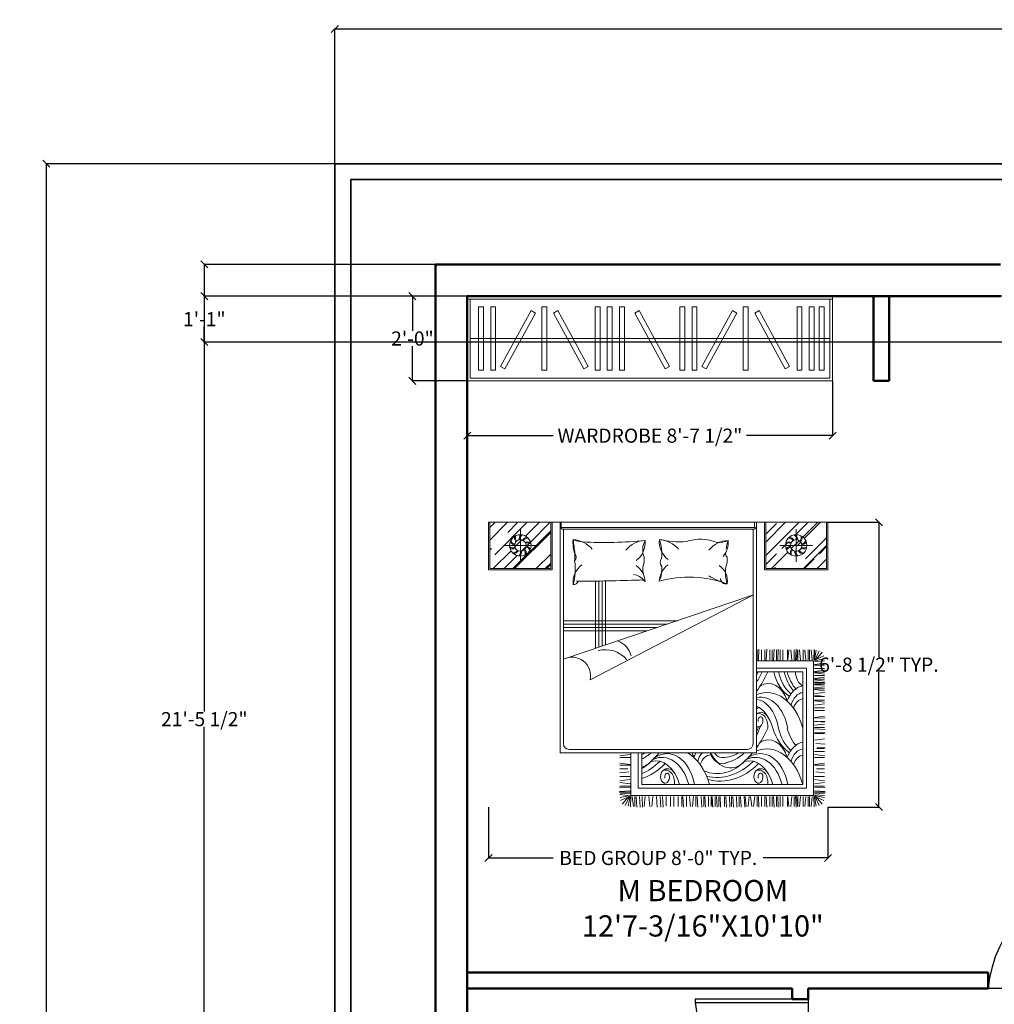
# Model space of a CAD drawing. Units: inches. Extents: x -317284 to 524, y -2236 to 1075.
# Tile 5 of 6: x -24 to 252, y 796 to 1075. Entities that reach past the tile are written whole.
import ezdxf

# ---------------------------------------------------------------- set-up
doc = ezdxf.new("R2010")
doc.units = ezdxf.units.IN
doc.header["$MEASUREMENT"] = 0
for name, color, linetype, lineweight in [('A-ANNO-DIMS', 2, 'Continuous', 18), ('A-AREA-IDEN', 7, 'Continuous', 18), ('A-DOOR', 4, 'Continuous', 25), ('A-FLOR-CASE', 8, 'Continuous', 20), ('A-FURN', 8, 'Continuous', 18), ('A-WALL', 7, 'Continuous', 50), ('C-PROP', 3, 'Continuous', 35)]:
    doc.layers.add(name, color=color, linetype=linetype, lineweight=lineweight)
doc.styles.get("Standard").update_dxf_attribs({"font": 'arial.ttf'})
doc.dimstyles.get("Standard").update_dxf_attribs({"dimtxt": 4, "dimasz": 2, "dimexe": 0.18, "dimexo": 0.0625, "dimgap": 0.09, "dimtad": 0, "dimtih": 1, "dimtoh": 1, "dimdec": 0, "dimzin": 0, "dimdsep": 46, "dimlunit": 4, "dimtxsty": 'Standard', "dimblk": 'OBLIQUE', "dimcen": 0.09, "dimadec": 0, "dimazin": 0, "dimtfac": 1, "dimtdec": 0, "dimtofl": 0, "dimtmove": 0, "dimatfit": 3, "dimldrblk": 'OBLIQUE', "dimfxl": 1, "dimtolj": 1, "dimtzin": 0, "dimarcsym": 0})

# ---------------------------------------------------------------- blocks, each defined once
blk = doc.blocks.new('SDFGHJK')
for p, q in [((282.73, 832.88), (281.73, 832.88)), ((281.73, 832.88), (281.73, 800.88)), ((282.73, 800.88), (282.73, 832.88)), ((282.73, 800.88), (250.73, 800.88))]:
    blk.add_line(p, q)
blk.add_arc((286.22, 797.51), 35.65, 97.2399, 174.5788)
blk = doc.blocks.new('A$C141F3920')
for p, q in [((600, 2590), (0, 2590)), ((0, 2590), (0, 0)), ((20, 0), (20, 2590)), ((600, 0), (600, 2590)), ((580, 2570), (20, 2570)), ((75, 2530.3), (75, 2495.3)), ((525, 2530.3), (75, 2530.3)), ((300, 20), (300, 2570)), ((525, 2495.3), (525, 2530.3)), ((580, 20), (580, 2570)), ((75, 2495.3), (525, 2495.3)), ((75, 2458.1), (75, 2423.1)), ((525, 2458.1), (75, 2458.1)), ((525, 2423.1), (525, 2458.1)), ((75, 2423.1), (525, 2423.1)), ((75, 2372.7), (75, 2337.7)), ((525, 2372.7), (75, 2372.7)), ((75, 2337.7), (525, 2337.7)), ((525, 2337.7), (525, 2372.7)), ((102.6, 2069.2), (497.4, 2285.1)), ((514.2, 2254.4), (119.4, 2038.5)), ((497.4, 2285.1), (514.2, 2254.4)), ((119.4, 2038.5), (102.6, 2069.2)), ((75, 1992), (75, 1957)), ((525, 1992), (75, 1992)), ((75, 1957), (525, 1957)), ((525, 1957), (525, 1992)), ((119.4, 1910.5), (102.6, 1879.8)), ((514.2, 1694.6), (119.4, 1910.5)), ((102.6, 1879.8), (497.4, 1663.9)), ((497.4, 1663.9), (514.2, 1694.6)), ((75, 1628.5), (75, 1593.5)), ((525, 1628.5), (75, 1628.5)), ((525, 1593.5), (525, 1628.5)), ((75, 1593.5), (525, 1593.5)), ((75, 1543.1), (75, 1508.1)), ((525, 1543.1), (75, 1543.1)), ((525, 1508.1), (525, 1543.1)), ((75, 1508.1), (525, 1508.1)), ((102.6, 1218.8), (497.4, 1434.8)), ((514.2, 1404), (119.4, 1188.1)), ((497.4, 1434.8), (514.2, 1404)), ((119.4, 1188.1), (102.6, 1218.8)), ((75, 1113.6), (75, 1078.6)), ((525, 1113.6), (75, 1113.6)), ((75, 1078.6), (525, 1078.6)), ((525, 1078.6), (525, 1113.6)), ((75, 1027.8), (75, 992.8)), ((525, 1027.8), (75, 1027.8)), ((75, 992.8), (525, 992.8)), ((525, 992.8), (525, 1027.8)), ((75, 942.3), (75, 907.3)), ((525, 942.3), (75, 942.3)), ((75, 907.3), (525, 907.3)), ((525, 907.3), (525, 942.3)), ((102.6, 641.9), (497.4, 857.9)), ((497.4, 857.9), (514.2, 827.2)), ((514.2, 827.2), (119.4, 611.2)), ((119.4, 611.2), (102.6, 641.9)), ((75, 564.8), (75, 529.8)), ((525, 564.8), (75, 564.8)), ((525, 529.8), (525, 564.8)), ((75, 529.8), (525, 529.8)), ((119.4, 483.3), (102.6, 452.6)), ((102.6, 452.6), (497.4, 236.7)), ((514.2, 267.4), (119.4, 483.3)), ((497.4, 236.7), (514.2, 267.4)), ((75, 201.3), (75, 166.3)), ((525, 201.3), (75, 201.3)), ((75, 166.3), (525, 166.3)), ((525, 166.3), (525, 201.3)), ((75, 115.8), (75, 80.8)), ((525, 115.8), (75, 115.8)), ((75, 80.8), (525, 80.8)), ((525, 80.8), (525, 115.8)), ((20, 20), (580, 20)), ((0, 0), (600, 0))]:
    blk.add_line(p, q)
blk = doc.blocks.new('A$C64B41DC1')
for p, q in [((0, 2.5079), (2.9903, 2.5079)), ((0, 2.0879), (0, 2.5079)), ((0.012, 2.4618), (0.0581, 2.5079)), ((0.012, 2.3515), (0.1684, 2.5079)), ((0.012, 2.0999), (0.012, 2.5079)), ((0.0543, 2.2213), (0.3409, 2.5079)), ((0.1689, 2.4179), (0.2589, 2.5079)), ((0.2157, 2.0999), (0.548, 2.4322)), ((0.2804, 2.1597), (0.2804, 2.4481)), ((0.3265, 2.386), (0.4484, 2.5079)), ((0.3699, 2.3332), (0.5445, 2.5079)), ((0.548, 2.5079), (0.548, 2.0999)), ((0.56, 2.5079), (0.56, 2.0879)), ((0.6301, 2.5079), (0.6301, 0.4779)), ((0.6401, 2.461), (0.6401, 2.5079)), ((0.6401, 2.5079), (2.344, 2.5079)), ((2.344, 2.461), (0.6401, 2.461)), ((0.6601, 2.4461), (1.4951, 2.4461)), ((0.6601, 2.4461), (0.6601, 0.5579)), ((1.4951, 2.4461), (0.6697, 2.4461)), ((2.3301, 2.4461), (1.4951, 2.4461)), ((2.3301, 0.5579), (2.3301, 2.4461)), ((2.344, 2.5079), (2.3601, 2.5079)), ((2.344, 2.5079), (2.344, 2.461)), ((2.3601, 2.5079), (2.3601, 2.4761)), ((2.3601, 0.4779), (2.3601, 2.5079)), ((2.4303, 2.5079), (2.4303, 2.0879)), ((2.4423, 2.5079), (2.4423, 2.0999)), ((2.4423, 2.3333), (2.6169, 2.5079)), ((2.4423, 2.2145), (2.7357, 2.5079)), ((2.4423, 2.404), (2.5354, 2.4971)), ((2.705, 2.398), (2.8149, 2.5079)), ((2.7099, 2.1597), (2.7099, 2.4481)), ((2.7691, 2.3772), (2.8998, 2.5079)), ((2.7819, 2.3646), (2.9252, 2.5079)), ((2.9783, 2.0999), (2.9783, 2.5079)), ((2.9903, 2.0879), (2.9903, 2.5079)), ((0.2299, 2.0999), (0.548, 2.418)), ((0.2311, 2.2906), (0.2937, 2.3532)), ((2.6674, 2.2756), (2.7382, 2.3464)), ((2.7914, 2.1846), (2.9783, 2.3715)), ((0.012, 2.261), (0.0275, 2.2765)), ((0.0404, 2.0999), (0.1982, 2.2578)), ((0.1362, 2.3039), (0.4246, 2.3039)), ((0.2905, 2.2539), (0.3304, 2.2938)), ((0.3405, 2.3039), (0.3605, 2.3238)), ((2.8541, 2.3039), (2.5657, 2.3039)), ((2.5849, 2.2779), (2.6158, 2.3088)), ((2.6158, 2.3088), (2.6313, 2.3243)), ((2.7249, 2.3076), (2.7512, 2.3339)), ((2.7746, 2.0999), (2.9783, 2.3036)), ((2.9144, 2.2312), (2.9783, 2.2951)), ((0.1365, 2.0999), (0.251, 2.2144)), ((0.4194, 2.0999), (0.548, 2.2285)), ((2.4423, 2.1353), (2.5382, 2.2312)), ((2.4918, 2.0999), (2.6366, 2.2447)), ((2.7831, 2.0999), (2.8678, 2.1846)), ((2.8962, 2.0999), (2.9783, 2.182)), ((0.56, 2.0879), (0, 2.0879)), ((0.548, 2.0999), (0.012, 2.0999)), ((0.4986, 2.0999), (0.548, 2.1493)), ((0.5127, 2.0999), (0.548, 2.1352)), ((2.4303, 2.0879), (2.9903, 2.0879)), ((2.4423, 2.0999), (2.9783, 2.0999)), ((2.5172, 2.0999), (2.5269, 2.1096)), ((0.9415, 1.9902), (0.9415, 1.3975)), ((0.9715, 1.9906), (0.9715, 1.4076)), ((1.0015, 1.991), (1.0015, 1.4177)), ((1.0315, 1.9916), (1.0315, 1.4279)), ((2.3349, 1.8678), (0.6613, 1.3029)), ((0.8956, 1.1191), (2.3349, 1.8678)), ((1.6636, 1.6412), (0.6601, 1.6412)), ((1.5748, 1.6112), (0.6601, 1.6112)), ((2.377, 1.295), (2.3822, 1.3891)), ((2.4451, 1.295), (2.4503, 1.3891)), ((2.5105, 1.295), (2.5157, 1.3891)), ((2.5471, 1.295), (2.5524, 1.3891)), ((2.7043, 1.295), (2.7095, 1.3891)), ((2.3665, 1.295), (2.3665, 1.3839)), ((2.4032, 1.295), (2.4032, 1.3839)), ((2.4346, 1.295), (2.4346, 1.3839)), ((2.4774, 1.2957), (2.4774, 1.3837)), ((2.5, 1.295), (2.5, 1.3839)), ((2.5367, 1.295), (2.5367, 1.3839)), ((2.5681, 1.295), (2.5681, 1.3839)), ((2.5918, 1.295), (2.5918, 1.3839)), ((2.6346, 1.2957), (2.6346, 1.3837)), ((2.6362, 1.2957), (2.6467, 1.3839)), ((2.6729, 1.295), (2.6624, 1.3839)), ((2.6938, 1.295), (2.6938, 1.3839)), ((2.7127, 1.2957), (2.7232, 1.3839)), ((2.7253, 1.295), (2.7253, 1.3839)), ((2.7494, 1.295), (2.7389, 1.3839)), ((2.7718, 1.295), (2.7718, 1.3839)), ((2.7959, 1.295), (2.7854, 1.3839)), ((2.8146, 1.2957), (2.8146, 1.3837)), ((2.8146, 1.2957), (2.8146, 1.3837)), ((2.8282, 1.295), (2.8282, 1.3839)), ((2.8282, 1.295), (2.8282, 1.3839)), ((2.8523, 1.295), (2.8418, 1.3839)), ((2.8523, 1.295), (2.8418, 1.3839)), ((2.8653, 1.2966), (2.8688, 1.3861)), ((2.8711, 1.2957), (2.8711, 1.3837)), ((2.8711, 1.2957), (2.8875, 1.3822)), ((2.8713, 1.2927), (2.954, 1.3315)), ((2.8717, 1.2884), (2.9588, 1.3058)), ((2.8765, 1.2958), (2.9132, 1.3758)), ((2.8893, 1.3011), (2.9394, 1.3636)), ((2.3601, 1.2873), (2.8639, 1.2873)), ((2.3601, 1.2233), (2.7999, 1.2233)), ((2.7999, 1.2233), (2.7999, 0.1658)), ((2.8639, 1.2873), (2.8639, 0.1018)), ((2.8716, 1.2565), (2.9605, 1.2669)), ((2.8716, 1.2212), (2.9605, 1.2212)), ((2.8723, 1.2489), (2.9603, 1.2489)), ((2.8744, 1.2817), (2.9603, 1.2869)), ((2.3601, 1.1913), (2.7679, 1.1912)), ((2.7679, 1.1912), (2.7679, 0.1978)), ((2.8716, 1.1947), (2.9605, 1.2052)), ((2.8716, 1.181), (2.9605, 1.1705)), ((2.8716, 1.1595), (2.9605, 1.1595)), ((2.8716, 1.133), (2.9605, 1.1435)), ((2.8723, 1.1872), (2.9603, 1.1872)), ((2.8716, 1.1193), (2.9605, 1.1088)), ((2.8716, 1.1035), (2.9605, 1.093)), ((2.8716, 1.0965), (2.9605, 1.0965)), ((2.8716, 1.086), (2.9657, 1.0913)), ((2.8716, 1.0756), (2.9605, 1.0756)), ((2.8716, 1.0491), (2.9605, 1.0596)), ((2.8723, 1.1255), (2.9603, 1.1255)), ((2.8723, 1.0858), (2.9605, 1.0753)), ((2.8723, 1.0416), (2.9603, 1.0416)), ((2.8716, 1.0354), (2.9605, 1.0249)), ((2.8723, 0.9987), (2.9605, 1.0092)), ((2.8723, 0.985), (2.9605, 0.9745)), ((2.8723, 0.9735), (2.9603, 0.9735)), ((2.8716, 0.9346), (2.9605, 0.9241)), ((2.8723, 0.9408), (2.9603, 0.9408)), ((2.8723, 0.8979), (2.9605, 0.9084)), ((2.8723, 0.8726), (2.9603, 0.8726)), ((2.8716, 0.7885), (2.9605, 0.799)), ((2.8716, 0.7818), (2.9657, 0.787)), ((2.8723, 0.8505), (2.9603, 0.8505)), ((2.8716, 0.7503), (2.9657, 0.7556)), ((2.8716, 0.7204), (2.9605, 0.7309)), ((2.8716, 0.6995), (2.9605, 0.6995)), ((2.8723, 0.7571), (2.9605, 0.7466)), ((2.8716, 0.689), (2.9657, 0.6838)), ((2.8716, 0.6576), (2.9657, 0.6523)), ((2.8716, 0.6471), (2.9605, 0.6471)), ((2.8716, 0.5903), (2.9605, 0.6007)), ((2.882, 0.5582), (2.9657, 0.5536)), ((2.8909, 0.5263), (2.9657, 0.5222)), ((0.6301, 0.4779), (2.3601, 0.4779)), ((0.7101, 0.5079), (2.2801, 0.5079)), ((1.2465, 0.4625), (1.1576, 0.452)), ((1.2465, 0.4365), (1.1577, 0.4365)), ((1.2542, 0.1018), (1.2542, 0.4779)), ((1.3182, 0.1658), (1.3182, 0.4779)), ((1.3502, 0.1978), (1.3502, 0.4779)), ((2.8716, 0.4877), (2.9603, 0.4877)), ((2.8716, 0.4625), (2.9605, 0.452)), ((2.8716, 0.4365), (2.9603, 0.4365)), ((2.8928, 0.5169), (2.9605, 0.5169)), ((1.2465, 0.3746), (1.1576, 0.3851)), ((1.2465, 0.3684), (1.1577, 0.3684)), ((2.8716, 0.3746), (2.9605, 0.3851)), ((2.8716, 0.3684), (2.9603, 0.3684)), ((1.2355, 0.3092), (1.1576, 0.3)), ((1.2285, 0.3357), (1.1577, 0.3357)), ((1.2457, 0.2676), (1.1577, 0.2676)), ((2.8723, 0.2676), (2.9603, 0.2676)), ((2.8826, 0.3092), (2.9605, 0.3)), ((2.8896, 0.3357), (2.9603, 0.3357)), ((1.2465, 0.1742), (1.1524, 0.169)), ((1.2457, 0.2423), (1.1576, 0.2319)), ((1.2465, 0.2057), (1.1576, 0.2161)), ((1.2465, 0.1847), (1.1576, 0.1847)), ((2.7679, 0.1978), (1.3502, 0.1978)), ((2.8716, 0.2057), (2.9605, 0.2161)), ((2.8716, 0.1847), (2.9605, 0.1847)), ((2.8716, 0.1742), (2.9657, 0.169)), ((2.8723, 0.2423), (2.9605, 0.2319)), ((1.2465, 0.1428), (1.1524, 0.1376)), ((1.2465, 0.1334), (1.1524, 0.1281)), ((1.2465, 0.1323), (1.1576, 0.1323)), ((1.2465, 0.1323), (1.1576, 0.1323)), ((1.2465, 0.1), (1.1576, 0.1105)), ((1.2465, 0.1229), (1.1588, 0.1168)), ((1.2464, 0.1007), (1.1592, 0.0833)), ((1.2468, 0.0964), (1.1641, 0.0576)), ((1.2288, 0.088), (1.1787, 0.0255)), ((1.2415, 0.0933), (1.2049, 0.0133)), ((1.247, 0.0934), (1.2306, 0.0069)), ((1.2527, 0.0925), (1.2493, 0.003)), ((2.8639, 0.1018), (1.2542, 0.1018)), ((1.2658, 0.0941), (1.2762, 0.0052)), ((1.2899, 0.0941), (1.2899, 0.0052)), ((1.2999, 0.0941), (1.3051, 0)), ((2.7999, 0.1658), (1.3182, 0.1658)), ((1.3313, 0.0941), (1.3365, 0)), ((1.3523, 0.0941), (1.3575, 0)), ((1.3804, 0.0941), (1.3699, 0.0052)), ((1.4119, 0.0934), (1.4223, 0.0052)), ((1.4485, 0.0941), (1.438, 0.0052)), ((1.48, 0.0941), (1.4852, 0)), ((1.5114, 0.0941), (1.5166, 0)), ((1.5323, 0.0941), (1.5376, 0)), ((1.5638, 0.0941), (1.5638, 0.0105)), ((1.6021, 0.0941), (1.6021, 0.0052)), ((1.6336, 0.0941), (1.6336, 0.0052)), ((1.6702, 0.0941), (1.6702, 0.0052)), ((1.7017, 0.0941), (1.7017, 0.0052)), ((1.7122, 0.0941), (1.7174, 0)), ((1.7445, 0.0934), (1.7445, 0.0054)), ((1.7698, 0.0934), (1.7803, 0.0052)), ((1.8065, 0.0941), (1.796, 0.0052)), ((1.8274, 0.0941), (1.8274, 0.0052)), ((1.8379, 0.0941), (1.8431, 0)), ((1.8746, 0.0941), (1.8798, 0)), ((1.8955, 0.0941), (1.8955, 0.0052)), ((1.906, 0.0941), (1.9113, 0)), ((1.9384, 0.0934), (1.9384, 0.0054)), ((1.9609, 0.0941), (1.9609, 0.0052)), ((1.9636, 0.0934), (1.9741, 0.0052)), ((1.9714, 0.0941), (1.9766, 0)), ((1.9976, 0.0941), (1.9976, 0.0052)), ((2.0081, 0.0941), (2.0133, 0)), ((2.029, 0.0941), (2.029, 0.0052)), ((2.0395, 0.0941), (2.0447, 0)), ((2.0797, 0.0941), (2.0797, 0.0052)), ((2.0902, 0.0941), (2.0954, 0)), ((2.1216, 0.0941), (2.1269, 0)), ((2.1412, 0.0941), (2.1412, 0.0052)), ((2.1517, 0.0941), (2.1569, 0)), ((2.1831, 0.0941), (2.1884, 0)), ((2.2093, 0.0941), (2.2093, 0.0052)), ((2.2198, 0.0941), (2.225, 0)), ((2.2512, 0.0941), (2.2565, 0)), ((2.2603, 0.0934), (2.2707, 0.0052)), ((2.2969, 0.0941), (2.2864, 0.0052)), ((2.3089, 0.0934), (2.3193, 0.0052)), ((2.3455, 0.0941), (2.3351, 0.0052)), ((2.3665, 0.0941), (2.3665, 0.0052)), ((2.377, 0.0941), (2.3822, 0)), ((2.4032, 0.0941), (2.4032, 0.0052)), ((2.4346, 0.0941), (2.4346, 0.0052)), ((2.4451, 0.0941), (2.4503, 0)), ((2.4774, 0.0934), (2.4774, 0.0054)), ((2.5, 0.0941), (2.5, 0.0052)), ((2.5105, 0.0941), (2.5157, 0)), ((2.5367, 0.0941), (2.5367, 0.0052)), ((2.5471, 0.0941), (2.5524, 0)), ((2.5681, 0.0941), (2.5681, 0.0052)), ((2.5918, 0.0941), (2.5918, 0.0052)), ((2.6346, 0.0934), (2.6346, 0.0054)), ((2.6362, 0.0934), (2.6467, 0.0052)), ((2.6729, 0.0941), (2.6624, 0.0052)), ((2.6938, 0.0941), (2.6938, 0.0052)), ((2.7043, 0.0941), (2.7095, 0)), ((2.7127, 0.0934), (2.7232, 0.0052)), ((2.7253, 0.0941), (2.7253, 0.0052)), ((2.7494, 0.0941), (2.7389, 0.0052)), ((2.7718, 0.0941), (2.7718, 0.0052)), ((2.7959, 0.0941), (2.7854, 0.0052)), ((2.8146, 0.0934), (2.8146, 0.0054)), ((2.8282, 0.0941), (2.8282, 0.0052)), ((2.8523, 0.0941), (2.8418, 0.0052)), ((2.8653, 0.0925), (2.8688, 0.003)), ((2.8711, 0.0934), (2.8875, 0.0069)), ((2.8713, 0.0964), (2.954, 0.0576)), ((2.8716, 0.1428), (2.9657, 0.1376)), ((2.8716, 0.1334), (2.9657, 0.1281)), ((2.8716, 0.1323), (2.9605, 0.1323)), ((2.8716, 0.1229), (2.9593, 0.1168)), ((2.8717, 0.1007), (2.9588, 0.0833)), ((2.8744, 0.1074), (2.9603, 0.1022)), ((2.8765, 0.0933), (2.9132, 0.0133)), ((2.8893, 0.088), (2.9394, 0.0255))]:
    blk.add_line(p, q)
at = {"ltscale": 10}
for p, q in [((1.4859, 1.5812), (0.6601, 1.5812)), ((1.397, 1.5512), (0.6601, 1.5512))]:
    blk.add_line(p, q, dxfattribs=at)
for centre, radius in [((0.2804, 2.3039), 0.0942), ((0.2804, 2.3039), 0.051), ((2.7099, 2.3039), 0.0942), ((2.7099, 2.3039), 0.051)]:
    blk.add_circle(centre, radius)
for centre, radius, start, end in [((0.6601, 2.4761), 0.03, 180, 270), ((2.3301, 2.4761), 0.03, 270, 0), ((0.2417, 2.3614), 0.0462, 196.30017, 256.53802), ((0.2887, 2.3745), 0.0605, 172.17003, 218.48975), ((0.2828, 2.3731), 0.0462, 160.30017, 220.53802), ((0.3286, 2.3561), 0.0605, 136.17003, 182.48975), ((0.3231, 2.3585), 0.0462, 124.30017, 184.53802), ((0.3501, 2.3178), 0.0605, 100.17003, 146.48975), ((0.347, 2.323), 0.0462, 88.30017, 148.53802), ((1.0526, 2.3302), 0.3085, 175.30484, 198.69419), ((-0.8702, 2.0941), 1.6364, 4.80985, 9.18918), ((0.8579, 2.6278), 0.2948, 247.51785, 264.26696), ((0.728, 2.111), 0.245, 40.4189, 85.9871), ((1.0164, 5.7096), 3.3803, 266.81337, 276.16021), ((1.3963, 2.1044), 0.245, 94.0129, 139.5811), ((1.1858, 2.3288), 0.1943, 306.5711, 5.88998), ((1.5348, 2.2652), 0.1767, 151.77364, 201.69827), ((1.6986, 2.3355), 0.1943, 174.11002, 233.4289), ((1.1481, 2.2311), 0.3783, 353.49469, 19.18669), ((1.6871, 3.192), 0.8561, 257.74383, 273.62843), ((1.4882, 2.111), 0.245, 40.4189, 85.9871), ((1.8674, 1.9709), 0.3878, 68.20259, 108.9817), ((2.1269, 2.1044), 0.245, 94.0129, 139.5811), ((2.0342, 2.4856), 0.1563, 261.59582, 298.90918), ((1.9165, 2.3288), 0.1943, 333.73715, 5.88998), ((2.6058, 2.2028), 0.517, 163.60457, 172.3273), ((2.6433, 2.323), 0.0462, 31.46198, 91.69983), ((2.6402, 2.3178), 0.0605, 33.51025, 79.82997), ((2.6672, 2.3585), 0.0462, 355.46198, 55.69983), ((2.6617, 2.3561), 0.0605, 357.51025, 43.82997), ((2.7075, 2.3731), 0.0462, 319.46198, 19.69983), ((2.7016, 2.3745), 0.0605, 321.51025, 7.82997), ((2.7486, 2.3614), 0.0462, 283.46198, 343.69983), ((0.2153, 2.3276), 0.0462, 232.30017, 292.53802), ((0.2158, 2.3336), 0.0605, 244.17003, 290.48975), ((0.2457, 2.3659), 0.0605, 208.17003, 254.48975), ((0.2138, 2.2848), 0.0462, 268.30017, 328.53802), ((0.2107, 2.29), 0.0605, 280.17003, 326.48975), ((0.2779, 2.2347), 0.0462, 340.30017, 40.53802), ((0.272, 2.2333), 0.0605, 352.17003, 38.48975), ((0.3449, 2.2742), 0.0605, 64.17003, 110.48975), ((0.3455, 2.2802), 0.0462, 52.30017, 112.53802), ((0.3191, 2.2464), 0.0462, 16.30017, 76.53802), ((0.3151, 2.2419), 0.0605, 28.17003, 74.48975), ((2.6448, 2.2802), 0.0462, 67.46198, 127.69983), ((2.6454, 2.2742), 0.0605, 69.51025, 115.82997), ((2.6752, 2.2419), 0.0605, 105.51025, 151.82997), ((2.6712, 2.2464), 0.0462, 103.46198, 163.69983), ((2.7182, 2.2333), 0.0605, 141.51025, 187.82997), ((2.7123, 2.2347), 0.0462, 139.46198, 199.69983), ((2.7796, 2.29), 0.0605, 213.51025, 259.82997), ((2.7765, 2.2848), 0.0462, 211.46198, 271.69983), ((2.7744, 2.3336), 0.0605, 249.51025, 295.82997), ((2.775, 2.3276), 0.0462, 247.46198, 307.69983), ((2.7446, 2.3659), 0.0605, 285.51025, 331.82997), ((0.2377, 2.2493), 0.0462, 304.30017, 4.53802), ((0.2322, 2.2517), 0.0605, 316.17003, 2.48975), ((0.2688, 2.0945), 0.4956, 344.0243, 8.70709), ((0.7274, 2.2013), 0.0446, 314.4736, 42.17134), ((-1.6008, 2.277), 2.3618, 357.39054, 358.88764), ((1.204, 2.1778), 0.1681, 337.01697, 7.53676), ((1.5671, 2.1546), 0.0547, 142.08329, 220.902), ((1.9165, 2.3288), 0.1943, 320.94042, 333.73715), ((2.1347, 2.2313), 0.0459, 165.35061, 223.26844), ((1.9346, 2.1778), 0.1681, 337.01697, 7.53676), ((2.7581, 2.2517), 0.0605, 177.51025, 223.82997), ((2.7526, 2.2493), 0.0462, 175.46198, 235.69983), ((0.9385, 1.978), 0.1943, 126.5711, 185.88998), ((1.1858, 1.9714), 0.1943, 4.31813, 53.4289), ((1.5415, 2.0969), 0.1834, 175.22328, 196.23004), ((1.7059, 1.9714), 0.204, 127.11975, 175.09005), ((1.1965, 2.0983), 0.3299, 343.79543, 3.55541), ((1.9394, 1.991), 0.1651, 351.26213, 55.75721), ((2.4617, 2.0719), 0.3745, 173.82958, 196.4356), ((0.7246, 18.8439), 16.8552, 270.17399, 272.05214), ((1.2687, 1.9248), 0.1223, 33.62799, 86.47438), ((1.3401, 1.9404), 0.0603, 49.09906, 101.37023), ((1.7676, 1.0629), 0.9631, 69.65065, 105.96307), ((2.2748, 2.5795), 0.6373, 238.34989, 254.31375), ((2.0911, 2.0123), 0.0478, 179.77267, 283.80184), ((0.7417, 2.0149), 0.057, 273.47085, 328.54118), ((0.728, 2.2025), 0.245, 274.0129, 278.34166), ((1.0747, 1.2871), 0.1871, 14.1863, 69.12121), ((0.7347, 1.1553), 0.1649, 347.31088, 116.44537), ((1.0274, 1.1334), 0.2527, 40.62904, 104.37123), ((0.7101, 0.5579), 0.05, 180, 270), ((2.2801, 0.5579), 0.05, 270, 0)]:
    blk.add_arc(centre, radius, start, end)
for centre, major_axis, ratio, start_param, end_param in [((1.9938, 1.6262), (0, -0.7531), 0.68, 0.797284, 0.954936), ((2.0643, 1.466), (0, -0.5322), 0.68, 7.239912, 7.311536), ((1.9052, 1.7397), (0, -0.9842), 0.68, 0.74745, 0.979724), ((2.7455, 1.3081), (0, 0.3614), 0.68, 1.900046, 2.742661), ((2.7868, 1.3081), (0, 0.3614), 0.68, 1.900046, 2.614747), ((2.8372, 1.3081), (0, 0.3614), 0.68, 1.900046, 2.479658), ((2.8607, 1.3211), (0, 0.3614), 0.68, 1.938265, 2.479658), ((2.8057, 1.2079), (0, -0.1524), 0.68, 4.821745, 5.895886), ((2.4513, 0.5069), (0, 0.502), 0.68, 5.095327, 6.553458), ((2.4665, 0.8216), (0, -0.2664), 0.68, 2.006169, 3.565187), ((2.7862, 0.8069), (0, -0.2615), 0.68, 3.244645, 4.205018), ((2.396, 0.6032), (0, 0.3641), 0.68, -1.3172, 0.145284), ((2.7784, 0.8289), (0, -0.1802), 0.68, 3.227058, 4.318474), ((2.7821, 0.7971), (0, -0.1589), 0.68, 3.272942, 4.229533), ((2.3507, 0.5642), (0.0073, 0.3819), 0.56205, -1.21172, -0.009991), ((2.2964, 0.5771), (0, -0.3263), 0.68, 1.938944, 2.850232), ((2.0403, 1.6015), (0, -0.8763), 0.68, 6.849801, 6.887077), ((2.4005, 0.7132), (0, -0.1214), 0.68, 2.284368, 3.652258), ((2.3834, 0.7081), (0, 0.1147), 0.68, 4.593909, 6.585576), ((2.3961, 0.7628), (0, -0.0317), 0.68, 1.462497, 5.046281), ((2.3774, 0.7653), (0, -0.0593), 0.68, 5.841311, 7.755362), ((1.9938, 1.1295), (-0.0678, 0.7439), 0.610498, 3.917146, 4.063997), ((2.0643, 0.9693), (0, -0.5322), 0.68, 7.239912, 7.336618), ((1.9052, 1.243), (0, -0.9842), 0.68, 0.74745, 0.979724), ((2.7455, 0.8114), (-0.0599, 0.3735), 0.695517, 1.775813, 2.548612), ((2.7868, 0.8114), (0, 0.3614), 0.68, 1.900046, 2.614747), ((2.8607, 0.8243), (0, 0.3614), 0.68, 1.938265, 2.479658), ((2.4665, 0.3249), (0, -0.2664), 0.68, 2.006169, 3.565187), ((2.4513, 0.0102), (0, 0.502), 0.68, 5.095327, 6.553458), ((2.7862, 0.3102), (0, -0.2615), 0.68, 3.244645, 4.205018), ((1.242, 0.9693), (0, -0.5322), 0.68, 6.586764, 6.677612), ((1.1714, 1.1295), (-0.1157, 0.7241), 0.59432, 3.291697, 3.50733), ((1.0828, 1.243), (0, -0.9842), 0.68, 0.565948, 0.680366), ((1.5283, 0.0674), (0, -0.3703), 0.68, 1.930561, 3.464283), ((1.5736, 0.1065), (0, 0.3641), 0.68, -1.3172, 0.476403), ((1.6289, 0.0102), (0, 0.502), 0.68, 6.655152, 6.661293), ((1.6289, 0.0102), (0, 0.502), 0.68, 5.095327, 5.911219), ((1.6442, 0.3249), (0, -0.2664), 0.68, 2.006169, 2.182797), ((1.9638, 0.3102), (0, -0.2615), 0.68, 4.015924, 4.205018), ((1.956, 0.3322), (0, -0.1802), 0.68, 3.770744, 4.318474), ((1.9597, 0.3004), (0, -0.1589), 0.68, 3.14258, 4.229533), ((2.0606, 0.5616), (0, -0.1803), 0.68, 5.194792, 5.929328), ((2.0606, 0.5616), (0, -0.1803), 0.68, 5.194792, 6.723255), ((2.1315, 0.6603), (0, -0.3155), 0.68, 5.328638, 6.949396), ((2.0549, 0.5656), (0, -0.1303), 0.68, 5.450951, 6.054641), ((2.0643, 0.9693), (0, -0.5322), 0.68, 6.20013, 6.677612), ((1.9938, 1.1295), (-0.0678, 0.7439), 0.610498, 3.199135, 3.592282), ((1.9052, 1.243), (0, -0.9842), 0.68, 0.565948, 0.680366), ((2.3507, 0.0674), (0, -0.3703), 0.68, 1.930561, 3.464283), ((2.396, 0.1065), (0, 0.3641), 0.68, -1.3172, 0.476403), ((2.4513, 0.0102), (0, 0.502), 0.68, 6.655152, 6.661293), ((2.7784, 0.3322), (0, -0.1802), 0.68, 3.227058, 4.318474), ((2.7821, 0.3004), (0, -0.1589), 0.68, 3.272942, 4.229533), ((1.1933, 0.9181), (0, -0.624), 0.68, 0.378672, 0.625379), ((1.3091, 0.6603), (0, -0.3155), 0.68, 6.475719, 6.949396), ((1.1911, 1.1066), (0, 0.8458), 0.68, 3.421828, 3.728616), ((1.2179, 1.1047), (0, -0.8763), 0.68, 6.507006, 6.887077), ((1.474, 0.0804), (0, -0.3263), 0.68, 1.938944, 3.339184), ((1.5781, 0.2165), (0, -0.1214), 0.68, 2.284368, 3.726131), ((2.0157, 0.9181), (0, -0.624), 0.68, -0.280078, 0.625379), ((2.0135, 1.1066), (0, 0.8458), 0.68, 2.978727, 3.728616), ((2.0403, 1.1047), (0, -0.8763), 0.68, 6.099302, 6.887077), ((2.2964, 0.0804), (0, -0.3263), 0.68, 1.938944, 3.339184), ((2.4005, 0.2165), (0, -0.1214), 0.68, 2.284368, 3.726131), ((1.555, 0.2685), (0, -0.0593), 0.68, 3.732151, 7.755362), ((1.561, 0.2114), (0, 0.1147), 0.68, 4.593909, 6.647252), ((1.5737, 0.2661), (0, -0.0317), 0.68, 1.462497, 5.046281), ((2.3774, 0.2685), (0, -0.0593), 0.68, 3.732151, 7.755362), ((2.3834, 0.2114), (0, 0.1147), 0.68, 4.593909, 6.647252), ((2.3961, 0.2661), (0, -0.0317), 0.68, 1.462497, 5.046281)]:
    blk.add_ellipse(centre, major_axis=major_axis, ratio=ratio, start_param=start_param, end_param=end_param)
blk = doc.blocks.new('_Oblique')
at = {"color": 0, "linetype": 'ByBlock', "lineweight": -2}
blk.add_line((-0.5, -0.5), (0.5, 0.5), dxfattribs=at)
blk = doc.blocks.new('*D14')
at = {"layer": 'A-ANNO-DIMS', "color": 0, "lineweight": -2, "transparency": 16777216}
for p, q in [((65.73, 1034.44), (65.73, 1072.72)), ((65.73, 1072.54), (263.52, 1072.54)), ((475.23, 1072.54), (277.44, 1072.54)), ((475.23, 1034.44), (475.23, 1072.72))]:
    blk.add_line(p, q, dxfattribs=at)
at = {"layer": 'Defpoints', "color": 0, "transparency": 16777216}
for p in [(475.23, 1072.54), (65.73, 1034.38), (475.23, 1034.38)]:
    blk.add_point(p, dxfattribs=at)
at = {"layer": 'A-ANNO-DIMS', "color": 0, "lineweight": -2, "transparency": 16777216, "xscale": 2, "yscale": 2, "zscale": 2, "rotation": 180}
blk.add_blockref('_Oblique', (65.73, 1072.54), dxfattribs=at)
at = {"layer": 'A-ANNO-DIMS', "color": 0, "lineweight": -2, "transparency": 16777216, "xscale": 2, "yscale": 2, "zscale": 2}
blk.add_blockref('_Oblique', (475.23, 1072.54), dxfattribs=at)
at = {"layer": 'A-ANNO-DIMS', "color": 0, "transparency": 16777216, "insert": (270.48, 1072.54), "char_height": 4, "attachment_point": 5}
blk.add_mtext('\\A1;34\'-2"', dxfattribs=at)
blk = doc.blocks.new('*D15')
at = {"layer": 'A-ANNO-DIMS', "color": 0, "lineweight": -2, "transparency": 16777216}
for p, q in [((65.66, 1034.38), (-16.14, 1034.38)), ((-15.96, 1034.38), (-15.96, 726.59)), ((-15.96, 414.53), (-15.96, 722.32)), ((65.66, 414.53), (-16.14, 414.53))]:
    blk.add_line(p, q, dxfattribs=at)
at = {"layer": 'Defpoints', "color": 0, "transparency": 16777216}
for p in [(-15.96, 1034.38), (65.73, 1034.38), (65.73, 414.53)]:
    blk.add_point(p, dxfattribs=at)
at = {"layer": 'A-ANNO-DIMS', "color": 0, "lineweight": -2, "transparency": 16777216, "xscale": 2, "yscale": 2, "zscale": 2}
for p, rotation in [((-15.96, 1034.38), 90), ((-15.96, 414.53), 270)]:
    blk.add_blockref('_Oblique', p, dxfattribs=dict(at, rotation=rotation))
at = {"layer": 'A-ANNO-DIMS', "color": 0, "transparency": 16777216, "insert": (-15.96, 724.45), "char_height": 4, "attachment_point": 5}
blk.add_mtext('\\A1;51\'-8"', dxfattribs=at)
blk = doc.blocks.new('*D23')
at = {"layer": 'A-ANNO-DIMS', "color": 0, "lineweight": -2, "transparency": 16777216}
for p, q in [((109.25, 852.18), (109.25, 837.64)), ((205.38, 852.18), (205.38, 837.64)), ((109.25, 837.82), (127.58, 837.82)), ((205.38, 837.82), (187.05, 837.82))]:
    blk.add_line(p, q, dxfattribs=at)
at = {"layer": 'Defpoints', "color": 0, "transparency": 16777216}
for p in [(109.25, 852.24), (205.38, 852.24), (205.38, 837.82)]:
    blk.add_point(p, dxfattribs=at)
at = {"layer": 'A-ANNO-DIMS', "color": 0, "lineweight": -2, "transparency": 16777216, "xscale": 2, "yscale": 2, "zscale": 2, "rotation": 180}
blk.add_blockref('_Oblique', (109.25, 837.82), dxfattribs=at)
at = {"layer": 'A-ANNO-DIMS', "color": 0, "lineweight": -2, "transparency": 16777216, "xscale": 2, "yscale": 2, "zscale": 2}
blk.add_blockref('_Oblique', (205.38, 837.82), dxfattribs=at)
at = {"layer": 'A-ANNO-DIMS', "color": 0, "transparency": 16777216, "insert": (157.31, 837.82), "char_height": 4, "attachment_point": 5}
blk.add_mtext('\\A1;BED GROUP 8\'-0" TYP.', dxfattribs=at)
blk = doc.blocks.new('*D24')
at = {"layer": 'A-ANNO-DIMS', "color": 0, "lineweight": -2, "transparency": 16777216}
for p, q in [((205.44, 932.86), (219.98, 932.86)), ((219.8, 932.86), (219.8, 894.71)), ((219.8, 852.24), (219.8, 890.39)), ((205.44, 852.24), (219.98, 852.24))]:
    blk.add_line(p, q, dxfattribs=at)
at = {"layer": 'Defpoints', "color": 0, "transparency": 16777216}
for p in [(205.38, 932.86), (219.8, 932.86), (205.38, 852.24)]:
    blk.add_point(p, dxfattribs=at)
at = {"layer": 'A-ANNO-DIMS', "color": 0, "lineweight": -2, "transparency": 16777216, "xscale": 2, "yscale": 2, "zscale": 2}
for p, rotation in [((219.8, 932.86), 90), ((219.8, 852.24), 270)]:
    blk.add_blockref('_Oblique', p, dxfattribs=dict(at, rotation=rotation))
at = {"layer": 'A-ANNO-DIMS', "color": 0, "transparency": 16777216, "insert": (219.8, 892.55), "char_height": 4, "attachment_point": 5}
blk.add_mtext('\\A1;6\'-8 1/2" TYP.', dxfattribs=at)
blk = doc.blocks.new('*D27')
at = {"layer": 'A-ANNO-DIMS', "color": 0, "lineweight": -2, "transparency": 16777216}
for p, q in [((103.23, 972.85), (103.23, 957.21)), ((206.68, 972.85), (206.68, 957.21)), ((103.23, 957.39), (127.58, 957.39)), ((206.68, 957.39), (182.33, 957.39))]:
    blk.add_line(p, q, dxfattribs=at)
at = {"layer": 'Defpoints', "color": 0, "transparency": 16777216}
for p in [(103.23, 972.91), (206.68, 972.91), (206.68, 957.39)]:
    blk.add_point(p, dxfattribs=at)
at = {"layer": 'A-ANNO-DIMS', "color": 0, "lineweight": -2, "transparency": 16777216, "xscale": 2, "yscale": 2, "zscale": 2, "rotation": 180}
blk.add_blockref('_Oblique', (103.23, 957.39), dxfattribs=at)
at = {"layer": 'A-ANNO-DIMS', "color": 0, "lineweight": -2, "transparency": 16777216, "xscale": 2, "yscale": 2, "zscale": 2}
blk.add_blockref('_Oblique', (206.68, 957.39), dxfattribs=at)
at = {"layer": 'A-ANNO-DIMS', "color": 0, "transparency": 16777216, "insert": (154.96, 957.39), "char_height": 4, "attachment_point": 5}
blk.add_mtext('\\A1;WARDROBE 8\'-7 1/2"', dxfattribs=at)
blk = doc.blocks.new('*D28')
at = {"layer": 'A-ANNO-DIMS', "color": 0, "lineweight": -2, "transparency": 16777216}
for p, q in [((103.16, 996.88), (87.53, 996.88)), ((87.71, 996.88), (87.71, 987.03)), ((87.71, 972.91), (87.71, 982.76)), ((103.16, 972.91), (87.53, 972.91))]:
    blk.add_line(p, q, dxfattribs=at)
at = {"layer": 'Defpoints', "color": 0, "transparency": 16777216}
for p in [(103.23, 996.88), (87.71, 972.91), (103.23, 972.91)]:
    blk.add_point(p, dxfattribs=at)
at = {"layer": 'A-ANNO-DIMS', "color": 0, "lineweight": -2, "transparency": 16777216, "xscale": 2, "yscale": 2, "zscale": 2}
for p, rotation in [((87.71, 996.88), 90), ((87.71, 972.91), 270)]:
    blk.add_blockref('_Oblique', p, dxfattribs=dict(at, rotation=rotation))
at = {"layer": 'A-ANNO-DIMS', "color": 0, "transparency": 16777216, "insert": (87.71, 984.9), "char_height": 4, "attachment_point": 5}
blk.add_mtext('\\A1;2\'-0"', dxfattribs=at)
blk = doc.blocks.new('*D33')
at = {"layer": 'A-ANNO-DIMS', "color": 0, "lineweight": -2, "transparency": 16777216}
for p, q in [((94.16, 1005.88), (28.6, 1005.88)), ((28.78, 1005.88), (28.78, 879.29)), ((28.78, 748.38), (28.78, 874.97)), ((94.16, 748.38), (28.6, 748.38))]:
    blk.add_line(p, q, dxfattribs=at)
at = {"layer": 'Defpoints', "color": 0, "transparency": 16777216}
for p in [(94.23, 1005.88), (28.78, 748.38), (94.23, 748.38)]:
    blk.add_point(p, dxfattribs=at)
at = {"layer": 'A-ANNO-DIMS', "color": 0, "lineweight": -2, "transparency": 16777216, "xscale": 2, "yscale": 2, "zscale": 2}
for p, rotation in [((28.78, 1005.88), 90), ((28.78, 748.38), 270)]:
    blk.add_blockref('_Oblique', p, dxfattribs=dict(at, rotation=rotation))
at = {"layer": 'A-ANNO-DIMS', "color": 0, "transparency": 16777216, "insert": (28.78, 877.13), "char_height": 4, "attachment_point": 5}
blk.add_mtext('\\A1;21\'-5 1/2"', dxfattribs=at)
blk = doc.blocks.new('*D53')
at = {"layer": 'A-ANNO-DIMS', "color": 0, "lineweight": -2, "transparency": 16777216}
for p, q in [((342.66, 996.88), (28.6, 996.88)), ((28.78, 996.88), (28.78, 992.48)), ((28.78, 983.88), (28.78, 988.28)), ((342.66, 983.88), (28.6, 983.88))]:
    blk.add_line(p, q, dxfattribs=at)
at = {"layer": 'Defpoints', "color": 0, "transparency": 16777216}
for p in [(342.73, 996.88), (28.78, 983.88), (342.73, 983.88)]:
    blk.add_point(p, dxfattribs=at)
at = {"layer": 'A-ANNO-DIMS', "color": 0, "lineweight": -2, "transparency": 16777216, "xscale": 2, "yscale": 2, "zscale": 2}
for p, rotation in [((28.78, 996.88), 90), ((28.78, 983.88), 270)]:
    blk.add_blockref('_Oblique', p, dxfattribs=dict(at, rotation=rotation))
at = {"layer": 'A-ANNO-DIMS', "color": 0, "transparency": 16777216, "insert": (28.78, 990.38), "char_height": 4, "attachment_point": 5}
blk.add_mtext('\\A1;1\'-1"', dxfattribs=at)

msp = doc.modelspace()

# ---------------------------------------------------------------- linework, layer by layer
at = {"layer": 'A-WALL'}
for p, q in [((103.23, 1005.88), (94.23, 1005.88)), ((94.23, 1005.88), (94.23, 996.88)), ((103.23, 1005.88), (254.23, 1005.88)), ((94.23, 996.88), (94.23, 876.88)), ((103.23, 996.88), (254.23, 996.88)), ((103.23, 996.88), (103.23, 876.88)), ((218.23, 972.88), (218.23, 996.88)), ((222.73, 996.88), (222.73, 972.88)), ((222.73, 972.88), (218.23, 972.88)), ((94.23, 876.88), (94.23, 748.38)), ((103.23, 876.88), (103.23, 805.38)), ((250.73, 805.38), (103.23, 805.38)), ((103.23, 805.38), (103.23, 752.88)), ((250.73, 805.38), (250.73, 800.88)), ((103.23, 800.88), (103.23, 752.88)), ((195.23, 800.88), (103.23, 800.88)), ((195.23, 800.88), (195.23, 797.88)), ((199.73, 800.88), (199.73, 797.88)), ((250.73, 800.88), (199.73, 800.88)), ((199.73, 797.88), (195.23, 797.88))]:
    msp.add_line(p, q, dxfattribs=at)
at = {"layer": 'C-PROP'}
for points in [[(475.23, 1034.38), (475.23, 414.53), (65.73, 414.53), (65.73, 1034.38)], [(470.73, 1029.88), (470.73, 419.03), (70.23, 419.03), (70.23, 1029.88)]]:
    msp.add_lwpolyline(points, close=True, dxfattribs=at)

# ---------------------------------------------------------------- block references
at = {"layer": 'A-DOOR'}
msp.add_blockref('SDFGHJK', (0, 0), dxfattribs=at)
at = {"layer": 'A-DOOR', "rotation": 90}
msp.add_blockref('SDFGHJK', (1000.61, 515.15), dxfattribs=at)
at = {"layer": 'A-FLOR-CASE', "xscale": 0.0399450428000942, "yscale": 0.0399450428000942, "zscale": 0.0399450428000942, "rotation": 270}
msp.add_blockref('A$C141F3920', (103.23, 996.88), dxfattribs=at)
at = {"layer": 'A-FURN', "xscale": 32.14740650668198, "yscale": 32.14740650668198, "zscale": 32.14740650668198}
msp.add_blockref('A$C64B41DC1', (109.25, 852.24), dxfattribs=at)

# ---------------------------------------------------------------- texts
at = {"layer": 'A-AREA-IDEN', "insert": (116.69, 831.58), "char_height": 6, "attachment_point": 1}
msp.add_mtext_dynamic_manual_height_columns('\\pxqc;M BEDROOM\\P12\'7-3/16"X10\'10"', width=106.4984, gutter_width=30, heights=[0], dxfattribs=at)

# ---------------------------------------------------------------- dimensions: what is measured, and where the dimension line sits
at = {"layer": 'A-ANNO-DIMS'}
dim = msp.add_linear_dim(base=(475.22661787, 1072.54228244), p1=(65.72661787, 1034.37939404), p2=(475.22661787, 1034.37939404), dimstyle='Standard', override={"dimclrd": 0, "dimclre": 0, "dimclrt": 0}, dxfattribs=at)
dim.commit()
dim.dimension.update_dxf_attribs({"geometry": '*D14', "text_midpoint": (270.47661787, 1072.54228244)})
for base, p1, p2, angle, override, picture, middle in [((-15.96, 1034.38), (65.73, 414.53), (65.73, 1034.38), 90, {"dimclrd": 0, "dimclre": 0, "dimclrt": 0}, '*D15', (-15.96, 724.45)), ((28.78, 748.38), (94.23, 1005.88), (94.23, 748.38), 90, {"dimdec": 1, "dimlfac": 1, "dimrnd": 0, "dimzin": 1, "dimdsep": 46, "dimlunit": 4, "dimfrac": 2}, '*D33', (28.78, 877.13)), ((28.78, 983.88), (342.73, 996.88), (342.73, 983.88), 90, {"dimdec": 1, "dimlfac": 1, "dimrnd": 0, "dimzin": 1, "dimdsep": 46, "dimlunit": 4, "dimfrac": 2}, '*D53', (28.78, 990.38)), ((87.71, 972.91), (103.23, 996.88), (103.23, 972.91), 270, {"dimdec": 1, "dimlfac": 1, "dimrnd": 0, "dimzin": 1, "dimdsep": 46, "dimlunit": 4, "dimfrac": 2}, '*D28', (87.71, 984.9))]:
    dim = msp.add_linear_dim(base=base, p1=p1, p2=p2, angle=angle, dimstyle='Standard', override=override, dxfattribs=at)
    dim.commit()
    dim.dimension.update_dxf_attribs({"geometry": picture, "text_midpoint": middle})
for base, p1, p2, text, picture, middle in [((206.6843, 957.3937), (103.2266, 972.9124), (206.6843, 972.9124), 'WARDROBE <>', '*D27', (154.9554, 957.3937)), ((205.38, 837.82), (109.25, 852.24), (205.38, 852.24), 'BED GROUP <> TYP.', '*D23', (157.31, 837.82))]:
    dim = msp.add_linear_dim(base=base, p1=p1, p2=p2, text=text, dimstyle='Standard', override={"dimdec": 1, "dimlfac": 1, "dimrnd": 0, "dimzin": 1, "dimdsep": 46, "dimlunit": 4, "dimfrac": 2}, dxfattribs=at)
    dim.commit()
    dim.dimension.update_dxf_attribs({"geometry": picture, "text_midpoint": middle})
dim = msp.add_linear_dim(base=(219.8, 932.86), p1=(205.38, 852.24), p2=(205.38, 932.86), angle=90, text='<> TYP.', dimstyle='Standard', override={"dimdec": 1, "dimlfac": 1, "dimrnd": 0, "dimzin": 1, "dimdsep": 46, "dimlunit": 4, "dimfrac": 2}, dxfattribs=at)
dim.commit()
dim.dimension.update_dxf_attribs({"geometry": '*D24', "text_midpoint": (219.8, 892.55)})

doc.saveas('drawing.dxf')
